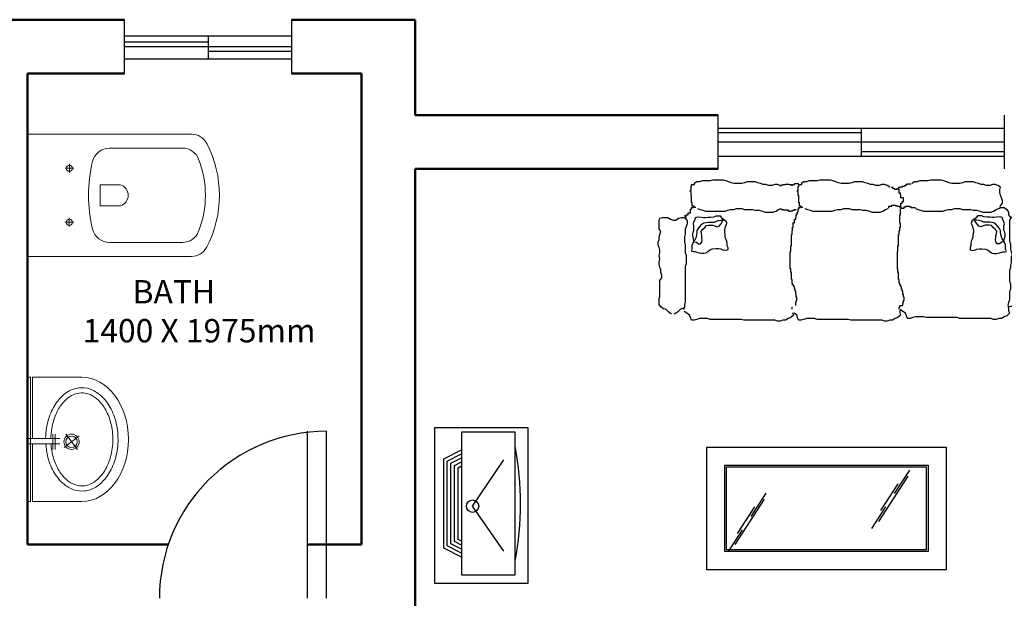
# Model space of a CAD drawing. Units: millimetres. Extents: x -857 to 54106, y -13666 to 13947.
# Tile 20 of 41: x 24413 to 28540, y 10779 to 13204. Entities that reach past the tile are written whole.
import ezdxf

# ---------------------------------------------------------------- set-up
doc = ezdxf.new("R2010")
doc.units = ezdxf.units.MM
for name, color, linetype, lineweight in [('A-AREA-IDEN', 3, 'Continuous', 18), ('A-DOOR', 1, 'Continuous', 25), ('A-FLOR-FIXT', 8, 'Continuous', 18), ('A-FURN', 21, 'Continuous', 18), ('A-GLAZ', 4, 'Continuous', 25), ('A-SANITARY FITTINGS', 25, 'Continuous', 15), ('A-WALL', 7, 'Continuous', 50)]:
    doc.layers.add(name, color=color, linetype=linetype, lineweight=lineweight)
doc.layers.add('TEFRIŞ', color=11, linetype='Continuous')
doc.styles.get("Standard").update_dxf_attribs({"font": 'arial.ttf'})

# ---------------------------------------------------------------- blocks, each defined once
blk = doc.blocks.new('A$C7d9d00ca')
at = {"layer": 'A-SANITARY FITTINGS'}
for p, q in [((0, 0), (-13.78, 0)), ((-13.78, -18.49), (-13.78, 0)), ((0, -18.49), (0, 0)), ((-9.94, -4.23), (-9.94, -5.23)), ((-3.84, -4.24), (-3.84, -5.24)), ((-10.42, -4.72), (-9.43, -4.72)), ((-3.36, -4.73), (-4.34, -4.73)), ((-12.2, -9.27), (-12.2, -17.48)), ((-1.57, -9.27), (-1.57, -17.48))]:
    blk.add_line(p, q, dxfattribs=at)
for points in [[(-8.08, -8.19), (-5.7, -8.19), (-5.7, -8.19), (-5.7, -10.48)], [(-8.08, -8.19), (-8.08, -10.48)]]:
    blk.add_lwpolyline(points, dxfattribs=at)
for centre in [(-9.94, -4.72), (-3.84, -4.73)]:
    blk.add_circle(centre, 0.342, dxfattribs=at)
for centre, radius, start, end in [((-10.24, -9.27), 1.97, 103.8652, 180), ((-6.89, -22.82), 15.93, 76.135, 103.8652), ((-3.54, -9.27), 1.97, 0.0003, 76.135), ((-6.89, -10.13), 1.24, 196.5098, 343.4902), ((-10.24, -17.48), 1.97, 180, 248.6555), ((-3.54, -17.48), 1.97, 291.3447, 0.0003), ((-11.81, -18.49), 1.97, 180, 242.8074), ((-1.97, -18.49), 1.97, 297.1926, 0), ((-6.89, -8.92), 11.16, 248.6555, 291.3447), ((-6.89, -8.92), 12.74, 242.8074, 297.1926)]:
    blk.add_arc(centre, radius, start, end, dxfattribs=at)
blk = doc.blocks.new('A$C0124305E')
at = {"layer": 'A-SANITARY FITTINGS'}
for p, q in [((-8.42, 16.01), (-0.8, 16.01)), ((-0.8, 7.08), (-0.8, 16.01)), ((-5.66, 7.68), (-8, 5.88)), ((-7.73, 7.95), (-5.93, 5.62)), ((-4.31, 5.61), (-4.31, 7.96)), ((-3.91, 5.61), (-3.91, 7.96)), ((0, 7.08), (-4.99, 7.08)), ((0, 6.28), (-4.99, 6.28)), ((-0.8, -3.19), (-0.8, 6.28)), ((-8.42, -3.19), (-0.8, -3.19))]:
    blk.add_line(p, q, dxfattribs=at)
blk.add_lwpolyline([(-0.5, 16.01), (0, 16.01), (0, -3.19), (-0.5, -3.19)], close=True, dxfattribs=at)
for radius in [1.18, 0.885]:
    blk.add_circle((-6.83, 6.78), radius, dxfattribs=at)
at = {"layer": 'A-SANITARY FITTINGS', "extrusion": (0, 0, -1)}
blk.add_ellipse((-8.42, 6.41), major_axis=(0, 9.6), ratio=0.75, start_param=3.141593, end_param=6.283185, dxfattribs=at)
at = {"layer": 'A-SANITARY FITTINGS'}
for points, knots in [([(-2.82, 6.28), (-2.82, 5.74), (-2.87, 5.2), (-3.1, 3.74), (-3.37, 2.86), (-4.09, 1.28), (-4.55, 0.6), (-5.56, -0.5), (-6.12, -0.92), (-7.25, -1.45), (-7.83, -1.58), (-8.98, -1.59), (-9.55, -1.46), (-10.69, -0.93), (-11.25, -0.52), (-12.27, 0.57), (-12.72, 1.25), (-13.45, 2.82), (-13.72, 3.71), (-14.02, 5.56), (-14.05, 6.52), (-13.88, 8.41), (-13.67, 9.32), (-13.04, 10.99), (-12.62, 11.73), (-11.66, 12.96), (-11.12, 13.45), (-10, 14.13), (-9.43, 14.32), (-8.28, 14.45), (-7.7, 14.39), (-6.56, 14), (-5.99, 13.66), (-4.93, 12.71), (-4.44, 12.09), (-3.62, 10.62), (-3.3, 9.78), (-2.96, 8.29), (-2.87, 7.69), (-2.84, 7.08)], [1.58652, 1.58652, 1.58652, 1.58652, 1.780321, 1.780321, 2.120053, 2.120053, 2.459785, 2.459785, 2.799517, 2.799517, 3.139249, 3.139249, 3.478981, 3.478981, 3.818713, 3.818713, 4.158445, 4.158445, 4.498177, 4.498177, 4.837909, 4.837909, 5.177641, 5.177641, 5.517373, 5.517373, 5.857105, 5.857105, 6.196837, 6.196837, 6.536569, 6.536569, 6.876301, 6.876301, 7.216033, 7.216033, 7.555765, 7.555765, 7.774364, 7.774364, 7.774364, 7.774364]), ([(-3.62, 6.29), (-3.62, 5.76), (-3.67, 5.23), (-3.88, 3.96), (-4.1, 3.23), (-4.65, 1.95), (-4.98, 1.39), (-5.72, 0.46), (-6.12, 0.1), (-6.92, -0.44), (-7.32, -0.61), (-8.11, -0.8), (-8.5, -0.81), (-9.28, -0.69), (-9.68, -0.55), (-10.48, -0.08), (-10.89, 0.24), (-11.67, 1.13), (-12.05, 1.7), (-12.66, 3.01), (-12.9, 3.76), (-13.2, 5.38), (-13.25, 6.28), (-13.13, 8.02), (-12.95, 8.88), (-12.42, 10.42), (-12.06, 11.12), (-11.23, 12.25), (-10.77, 12.7), (-9.92, 13.26), (-9.53, 13.43), (-8.78, 13.62), (-8.41, 13.64), (-7.66, 13.54), (-7.28, 13.42), (-6.51, 13.02), (-6.12, 12.73), (-5.35, 11.95), (-4.97, 11.43), (-4.34, 10.23), (-4.08, 9.54), (-3.76, 8.24), (-3.67, 7.64), (-3.63, 7.03)], [1.58652, 1.58652, 1.58652, 1.58652, 1.790653, 1.790653, 2.093007, 2.093007, 2.384527, 2.384527, 2.676047, 2.676047, 2.967567, 2.967567, 3.259087, 3.259087, 3.550608, 3.550608, 3.842128, 3.842128, 4.155456, 4.155456, 4.468784, 4.468784, 4.806699, 4.806699, 5.144614, 5.144614, 5.482529, 5.482529, 5.820444, 5.820444, 6.099515, 6.099515, 6.378586, 6.378586, 6.657656, 6.657656, 6.936727, 6.936727, 7.23864, 7.23864, 7.540552, 7.540552, 7.774364, 7.774364, 7.774364, 7.774364])]:
    blk.add_open_spline(points, degree=3, knots=knots, dxfattribs=at)
blk = doc.blocks.new('27')
at = {"layer": 'TEFRIŞ'}
for p, q in [((-1750.11, -460.72), (-1775.76, -443.38)), ((-1725.16, -443.38), (-1750.11, -460.72))]:
    blk.add_line(p, q, dxfattribs=at)
for points in [[(-1707.18, -481.65), (-1793.65, -481.65), (-1793.65, -429.97), (-1707.18, -429.97)], [(-1791.19, -466.78), (-1711.98, -466.78), (-1711.98, -437.07), (-1791.19, -437.07)]]:
    blk.add_lwpolyline(points, close=True, dxfattribs=at)
for points in [[(-1721.88, -466.78), (-1726.83, -476.68), (-1776.34, -476.68), (-1781.29, -466.78)], [(-1724.1, -466.78), (-1728.06, -474.7), (-1775.12, -474.7), (-1779.08, -466.78)], [(-1726.31, -466.78), (-1729.28, -472.72), (-1773.89, -472.72), (-1776.86, -466.78)], [(-1728.53, -466.78), (-1730.51, -470.74), (-1772.67, -470.74), (-1774.65, -466.78)], [(-1730.74, -466.78), (-1731.73, -468.76), (-1771.44, -468.76), (-1772.43, -466.78)]]:
    blk.add_lwpolyline(points, dxfattribs=at)
blk.add_circle((-1750.11, -460.72), 3.43, dxfattribs=at)
blk.add_arc((-1751.43, -604.56), 170.46, 79.2853, 100.7147, dxfattribs=at)
blk = doc.blocks.new('24')
at = {"layer": 'TEFRIŞ'}
for p, q in [((-1851.9, -153.78), (-1851.9, -152.78)), ((-1851.9, -152.78), (-1850.24, -152.78)), ((-1849.09, -151.25), (-1850.56, -152.23)), ((-1850.24, -152.78), (-1850.24, -152.11)), ((-1847.61, -151.25), (-1849.09, -151.25)), ((-1846.13, -150.75), (-1847.61, -151.25)), ((-1841.7, -150.75), (-1846.13, -150.75)), ((-1840.23, -150.26), (-1841.7, -150.75)), ((-1834.32, -150.26), (-1840.23, -150.26)), ((-1832.84, -150.75), (-1834.32, -150.26)), ((-1831.36, -151.25), (-1832.84, -150.75)), ((-1829.89, -151.74), (-1831.36, -151.25)), ((-1828.41, -152.23), (-1829.89, -151.74)), ((-1823.98, -152.23), (-1828.41, -152.23)), ((-1822.5, -151.74), (-1823.98, -152.23)), ((-1821.03, -151.25), (-1822.5, -151.74)), ((-1816.6, -151.25), (-1821.03, -151.25)), ((-1815.12, -151.74), (-1816.6, -151.25)), ((-1813.64, -152.23), (-1815.12, -151.74)), ((-1812.17, -152.72), (-1813.64, -152.23)), ((-1810.69, -152.72), (-1812.17, -152.72)), ((-1809.21, -153.21), (-1810.69, -152.72)), ((-1805.77, -152.72), (-1807.24, -153.21)), ((-1804.29, -152.72), (-1805.77, -152.72)), ((-1802.81, -153.21), (-1804.29, -152.72)), ((-1801, -152.88), (-1801, -152.68)), ((-1801, -152.68), (-1800, -152.68)), ((-1800, -152.68), (-1800, -152.48)), ((-1800, -152.48), (-1797.79, -152.48)), ((-1797.79, -152.48), (-1797.79, -152.68)), ((-1797.79, -152.68), (-1796.79, -152.68)), ((-1796.79, -152.68), (-1796.79, -153.08)), ((-1795.78, -153.08), (-1795.78, -152.68)), ((-1795.78, -152.68), (-1794.78, -152.68)), ((-1794.78, -152.68), (-1794.78, -152.08)), ((-1794.78, -152.08), (-1792.77, -152.08)), ((-1792.77, -152.08), (-1792.77, -152.68)), ((-1792.77, -152.68), (-1792.57, -152.68)), ((-1792.5, -152.78), (-1790.84, -152.78)), ((-1792.5, -153.78), (-1792.5, -152.78)), ((-1789.69, -151.25), (-1791.16, -152.23)), ((-1790.84, -152.78), (-1790.84, -152.11)), ((-1788.21, -151.25), (-1789.69, -151.25)), ((-1786.73, -150.75), (-1788.21, -151.25)), ((-1782.3, -150.75), (-1786.73, -150.75)), ((-1780.83, -150.26), (-1782.3, -150.75)), ((-1774.92, -150.26), (-1780.83, -150.26)), ((-1773.44, -150.75), (-1774.92, -150.26)), ((-1771.96, -151.25), (-1773.44, -150.75)), ((-1770.49, -151.74), (-1771.96, -151.25)), ((-1769.01, -152.23), (-1770.49, -151.74)), ((-1764.58, -152.23), (-1769.01, -152.23)), ((-1763.1, -151.74), (-1764.58, -152.23)), ((-1761.63, -151.25), (-1763.1, -151.74)), ((-1757.2, -151.25), (-1761.63, -151.25)), ((-1755.72, -151.74), (-1757.2, -151.25)), ((-1754.24, -152.23), (-1755.72, -151.74)), ((-1752.77, -152.72), (-1754.24, -152.23)), ((-1751.29, -152.72), (-1752.77, -152.72)), ((-1749.81, -153.21), (-1751.29, -152.72)), ((-1746.37, -152.72), (-1747.84, -153.21)), ((-1744.89, -152.72), (-1746.37, -152.72)), ((-1743.41, -153.21), (-1744.89, -152.72)), ((-1733.14, -152.78), (-1733.14, -153.45)), ((-1732.14, -152.78), (-1733.14, -152.78)), ((-1732.14, -152.45), (-1732.14, -152.78)), ((-1730.14, -152.45), (-1732.14, -152.45)), ((-1728.32, -151.25), (-1729.8, -152.23)), ((-1726.85, -151.25), (-1728.32, -151.25)), ((-1725.37, -150.75), (-1726.85, -151.25)), ((-1720.94, -150.75), (-1725.37, -150.75)), ((-1719.46, -150.26), (-1720.94, -150.75)), ((-1713.56, -150.26), (-1719.46, -150.26)), ((-1712.08, -150.75), (-1713.56, -150.26)), ((-1710.6, -151.25), (-1712.08, -150.75)), ((-1709.12, -151.74), (-1710.6, -151.25)), ((-1707.65, -152.23), (-1709.12, -151.74)), ((-1703.22, -152.23), (-1707.65, -152.23)), ((-1701.74, -151.74), (-1703.22, -152.23)), ((-1700.26, -151.25), (-1701.74, -151.74)), ((-1695.83, -151.25), (-1700.26, -151.25)), ((-1694.36, -151.74), (-1695.83, -151.25)), ((-1692.88, -152.23), (-1694.36, -151.74)), ((-1691.4, -152.72), (-1692.88, -152.23)), ((-1689.93, -152.72), (-1691.4, -152.72)), ((-1688.45, -153.21), (-1689.93, -152.72)), ((-1685, -152.72), (-1686.48, -153.21)), ((-1683.53, -152.72), (-1685, -152.72)), ((-1682.05, -153.21), (-1683.53, -152.72)), ((-1852.57, -156.78), (-1852.57, -155.78)), ((-1852.57, -155.78), (-1852.24, -155.78)), ((-1852.24, -156.78), (-1852.57, -156.78)), ((-1852.24, -155.78), (-1852.24, -153.78)), ((-1852.24, -153.78), (-1851.9, -153.78)), ((-1852.24, -158.78), (-1852.24, -156.78)), ((-1807.24, -153.21), (-1809.21, -153.21)), ((-1803.01, -153.28), (-1802.01, -153.28)), ((-1802.01, -153.28), (-1802.01, -152.88)), ((-1802.01, -152.88), (-1801, -152.88)), ((-1796.79, -153.08), (-1795.78, -153.08)), ((-1793.17, -155.78), (-1792.84, -155.78)), ((-1793.17, -156.78), (-1793.17, -155.78)), ((-1792.84, -156.78), (-1793.17, -156.78)), ((-1792.84, -155.78), (-1792.84, -153.78)), ((-1792.84, -153.78), (-1792.5, -153.78)), ((-1792.84, -158.78), (-1792.84, -156.78)), ((-1747.84, -153.21), (-1749.81, -153.21)), ((-1741.94, -154.2), (-1743.41, -153.21)), ((-1741.14, -154.45), (-1741.14, -154.11)), ((-1740.14, -154.45), (-1741.14, -154.45)), ((-1740.14, -155.11), (-1740.14, -154.45)), ((-1739.14, -155.11), (-1740.14, -155.11)), ((-1739.14, -155.45), (-1739.14, -155.11)), ((-1738.14, -155.45), (-1739.14, -155.45)), ((-1738.14, -155.11), (-1738.14, -155.45)), ((-1737.14, -155.11), (-1738.14, -155.11)), ((-1737.14, -154.45), (-1737.14, -155.11)), ((-1736.14, -154.45), (-1737.14, -154.45)), ((-1737.14, -155.45), (-1737.14, -155.11)), ((-1736.81, -155.45), (-1737.14, -155.45)), ((-1736.81, -157.45), (-1736.81, -155.45)), ((-1736.14, -157.45), (-1736.81, -157.45)), ((-1735.14, -154.11), (-1736.14, -154.11)), ((-1736.14, -154.11), (-1736.14, -154.45)), ((-1736.14, -158.45), (-1736.14, -157.45)), ((-1735.14, -153.78), (-1735.14, -154.11)), ((-1734.14, -153.78), (-1735.14, -153.78)), ((-1734.14, -153.45), (-1734.14, -153.78)), ((-1733.14, -153.45), (-1734.14, -153.45)), ((-1686.48, -153.21), (-1688.45, -153.21)), ((-1680.57, -154.2), (-1682.05, -153.21)), ((-1681.06, -155.67), (-1680.57, -154.2)), ((-1681.06, -157.15), (-1681.06, -155.67)), ((-1680.57, -158.63), (-1681.06, -157.15)), ((-1851.9, -158.78), (-1852.24, -158.78)), ((-1851.9, -162.78), (-1851.9, -158.78)), ((-1851.57, -162.78), (-1851.9, -162.78)), ((-1851.57, -164.78), (-1851.57, -162.78)), ((-1792.5, -158.78), (-1792.84, -158.78)), ((-1792.5, -162.78), (-1792.5, -158.78)), ((-1792.17, -162.78), (-1792.5, -162.78)), ((-1792.17, -164.78), (-1792.17, -162.78)), ((-1735.81, -158.45), (-1736.14, -158.45)), ((-1735.81, -160.11), (-1735.81, -158.45)), ((-1734.48, -160.11), (-1735.81, -160.11)), ((-1735.81, -163.11), (-1735.14, -163.11)), ((-1735.81, -165.11), (-1735.81, -163.11)), ((-1735.14, -162.11), (-1734.48, -162.11)), ((-1735.14, -163.11), (-1735.14, -162.11)), ((-1734.48, -162.11), (-1734.48, -160.11)), ((-1680.08, -160.1), (-1680.57, -158.63)), ((-1680.57, -164.53), (-1679.59, -163.05)), ((-1679.59, -161.58), (-1680.08, -160.1)), ((-1679.59, -163.05), (-1679.59, -161.58)), ((-1853.9, -169.44), (-1853.9, -168.44)), ((-1853.9, -168.44), (-1852.57, -168.44)), ((-1852.57, -168.44), (-1852.57, -166.44)), ((-1852.57, -166.44), (-1851.9, -166.44)), ((-1851.9, -166.44), (-1851.9, -165.44)), ((-1851.9, -165.44), (-1850.9, -165.44)), ((-1850.57, -164.78), (-1851.57, -164.78)), ((-1850.9, -165.44), (-1850.9, -164.78)), ((-1850.57, -165.44), (-1850.57, -164.78)), ((-1849.57, -165.44), (-1850.57, -165.44)), ((-1848.59, -166), (-1847.12, -166.5)), ((-1847.12, -166.5), (-1845.64, -166.99)), ((-1845.64, -166.99), (-1844.16, -167.48)), ((-1844.16, -167.48), (-1833.33, -167.48)), ((-1833.33, -167.48), (-1831.86, -166.99)), ((-1831.86, -166.99), (-1830.38, -166.5)), ((-1830.38, -166.5), (-1828.41, -166.5)), ((-1828.41, -166.5), (-1826.93, -166)), ((-1826.93, -166), (-1823.98, -166)), ((-1823.98, -166), (-1822.5, -166.5)), ((-1822.5, -166.5), (-1818.07, -166.5)), ((-1818.07, -166.5), (-1816.6, -166.99)), ((-1816.6, -166.99), (-1814.63, -166.99)), ((-1814.63, -166.99), (-1812.66, -167.48)), ((-1812.66, -167.48), (-1811.18, -167.97)), ((-1811.18, -167.97), (-1806.75, -167.97)), ((-1806.75, -167.97), (-1805.27, -167.48)), ((-1805.27, -167.48), (-1803.8, -166.5)), ((-1803.8, -166.5), (-1802.32, -166)), ((-1802.41, -166.32), (-1802.41, -165.92)), ((-1802.01, -166.32), (-1802.41, -166.32)), ((-1802.01, -166.72), (-1802.01, -166.32)), ((-1801, -166.72), (-1802.01, -166.72)), ((-1801, -166.92), (-1801, -166.72)), ((-1798.99, -166.92), (-1801, -166.92)), ((-1798.99, -167.12), (-1798.99, -166.92)), ((-1797.99, -167.12), (-1798.99, -167.12)), ((-1797.99, -167.72), (-1797.99, -167.12)), ((-1796.99, -167.72), (-1797.99, -167.72)), ((-1795.98, -167.52), (-1796.99, -167.52)), ((-1796.99, -167.52), (-1796.99, -167.72)), ((-1794.98, -167.12), (-1795.98, -167.12)), ((-1795.98, -167.12), (-1795.98, -167.52)), ((-1793.98, -166.72), (-1794.98, -166.72)), ((-1794.98, -166.72), (-1794.98, -167.12)), ((-1793.78, -169.93), (-1793.78, -168.92)), ((-1793.78, -168.92), (-1793.18, -168.92)), ((-1793.18, -168.92), (-1793.18, -167.92)), ((-1793.18, -167.92), (-1792.77, -167.92)), ((-1793.17, -166.44), (-1792.5, -166.44)), ((-1792.77, -167.92), (-1792.77, -166.32)), ((-1792.5, -165.44), (-1791.5, -165.44)), ((-1792.5, -166.44), (-1792.5, -165.44)), ((-1791.17, -164.78), (-1792.17, -164.78)), ((-1791.5, -165.44), (-1791.5, -164.78)), ((-1791.17, -165.44), (-1791.17, -164.78)), ((-1790.17, -165.44), (-1791.17, -165.44)), ((-1789.19, -166), (-1787.72, -166.5)), ((-1787.72, -166.5), (-1786.24, -166.99)), ((-1786.24, -166.99), (-1784.76, -167.48)), ((-1784.76, -167.48), (-1773.93, -167.48)), ((-1773.93, -167.48), (-1772.46, -166.99)), ((-1772.46, -166.99), (-1770.98, -166.5)), ((-1770.98, -166.5), (-1769.01, -166.5)), ((-1769.01, -166.5), (-1767.53, -166)), ((-1767.53, -166), (-1764.58, -166)), ((-1764.58, -166), (-1763.1, -166.5)), ((-1763.1, -166.5), (-1758.67, -166.5)), ((-1758.67, -166.5), (-1757.2, -166.99)), ((-1757.2, -166.99), (-1755.23, -166.99)), ((-1755.23, -166.99), (-1753.26, -167.48)), ((-1753.26, -167.48), (-1751.78, -167.97)), ((-1751.78, -167.97), (-1747.35, -167.97)), ((-1747.35, -167.97), (-1745.87, -167.48)), ((-1745.87, -167.48), (-1744.4, -166.5)), ((-1744.4, -166.5), (-1742.92, -166)), ((-1742.48, -164.78), (-1740.81, -164.78)), ((-1742.48, -165.78), (-1742.48, -164.78)), ((-1740.81, -164.11), (-1738.81, -164.11)), ((-1740.81, -164.78), (-1740.81, -164.11)), ((-1738.81, -164.11), (-1738.81, -164.45)), ((-1738.81, -164.45), (-1737.81, -164.45)), ((-1737.81, -164.45), (-1737.81, -164.78)), ((-1737.81, -164.78), (-1736.81, -164.78)), ((-1736.81, -164.78), (-1736.81, -165.11)), ((-1736.81, -165.11), (-1735.81, -165.11)), ((-1735.81, -165.44), (-1736.14, -165.44)), ((-1736.14, -165.78), (-1734.14, -165.78)), ((-1736.14, -166.11), (-1735.81, -166.11)), ((-1736.14, -169.44), (-1736.14, -166.11)), ((-1735.81, -165.11), (-1735.81, -165.44)), ((-1734.14, -165.11), (-1733.14, -165.11)), ((-1734.14, -165.78), (-1734.14, -165.11)), ((-1733.14, -164.78), (-1731.14, -164.78)), ((-1733.14, -165.11), (-1733.14, -164.78)), ((-1731.14, -164.78), (-1731.14, -165.11)), ((-1731.14, -165.11), (-1730.14, -165.11)), ((-1730.14, -165.11), (-1730.14, -165.44)), ((-1730.14, -165.44), (-1727.81, -165.44)), ((-1727.83, -166), (-1726.35, -166.5)), ((-1726.35, -166.5), (-1724.88, -166.99)), ((-1724.88, -166.99), (-1723.4, -167.48)), ((-1723.4, -167.48), (-1712.57, -167.48)), ((-1712.57, -167.48), (-1711.09, -166.99)), ((-1711.09, -166.99), (-1709.62, -166.5)), ((-1709.62, -166.5), (-1707.65, -166.5)), ((-1707.65, -166.5), (-1706.17, -166)), ((-1706.17, -166), (-1703.22, -166)), ((-1703.22, -166), (-1701.74, -166.5)), ((-1701.74, -166.5), (-1697.31, -166.5)), ((-1697.31, -166.5), (-1695.83, -166.99)), ((-1695.83, -166.99), (-1693.86, -166.99)), ((-1693.86, -166.99), (-1691.89, -167.48)), ((-1691.89, -167.48), (-1690.42, -167.97)), ((-1690.42, -167.97), (-1685.99, -167.97)), ((-1685.99, -167.97), (-1684.51, -167.48)), ((-1684.51, -167.48), (-1683.03, -166.5)), ((-1683.03, -166.5), (-1681.56, -166)), ((-1681.56, -166), (-1680.08, -165.51)), ((-1681.06, -166), (-1680.57, -164.53)), ((-1680.08, -165.51), (-1678.6, -165.51)), ((-1678.6, -165.51), (-1677.13, -166.5)), ((-1677.13, -166.5), (-1676.14, -167.97)), ((-1676.14, -167.97), (-1676.14, -169.45)), ((-1869.99, -172.89), (-1869.5, -171.42)), ((-1869.99, -177.32), (-1869.99, -172.89)), ((-1869.5, -171.42), (-1868.02, -170.92)), ((-1868.02, -170.92), (-1865.07, -170.92)), ((-1865.07, -170.92), (-1863.59, -171.91)), ((-1863.59, -171.91), (-1862.11, -172.4)), ((-1862.11, -172.4), (-1860.63, -172.4)), ((-1860.63, -172.4), (-1859.16, -171.42)), ((-1859.16, -171.42), (-1857.68, -170.92)), ((-1857.68, -170.92), (-1856.2, -170.92)), ((-1856.2, -170.92), (-1854.73, -171.42)), ((-1855.22, -171.42), (-1855.71, -169.94)), ((-1854.24, -172.89), (-1855.22, -171.42)), ((-1854.9, -169.44), (-1853.9, -169.44)), ((-1854.9, -170.78), (-1854.9, -169.44)), ((-1854.73, -175.84), (-1854.24, -174.37)), ((-1854.24, -174.37), (-1854.24, -172.89)), ((-1850.85, -174.48), (-1850.62, -173.32)), ((-1850.62, -175.64), (-1850.85, -174.48)), ((-1850.62, -173.32), (-1849.92, -172.16)), ((-1849.92, -172.16), (-1849.69, -171)), ((-1849.69, -171), (-1848.53, -170.54)), ((-1848.53, -170.54), (-1846.44, -170.77)), ((-1847.14, -175.87), (-1846.21, -174.71)), ((-1846.44, -170.77), (-1845.28, -171)), ((-1846.21, -174.71), (-1845.05, -174.01)), ((-1845.28, -171), (-1844.12, -171)), ((-1845.05, -174.01), (-1843.89, -173.78)), ((-1844.12, -171), (-1842.73, -170.77)), ((-1843.89, -173.78), (-1842.73, -173.55)), ((-1842.73, -170.77), (-1841.34, -170.77)), ((-1842.73, -173.55), (-1839.25, -173.55)), ((-1841.34, -170.77), (-1839.48, -170.54)), ((-1839.48, -170.54), (-1838.32, -170.07)), ((-1839.25, -173.55), (-1838.09, -173.09)), ((-1838.32, -170.07), (-1836, -170.07)), ((-1838.09, -173.09), (-1836.93, -172.62)), ((-1836.93, -172.62), (-1835.54, -172.39)), ((-1836.7, -175.87), (-1835.77, -174.71)), ((-1836, -170.07), (-1835.31, -171.23)), ((-1835.77, -174.71), (-1835.08, -173.55)), ((-1835.54, -172.39), (-1834.38, -172.16)), ((-1835.31, -171.23), (-1833.92, -172.16)), ((-1835.08, -173.55), (-1834.38, -172.39)), ((-1834.38, -172.39), (-1834.15, -171.93)), ((-1833.92, -172.16), (-1832.76, -173.09)), ((-1832.52, -174.25), (-1832.99, -175.4)), ((-1832.76, -173.09), (-1832.52, -174.25)), ((-1795.54, -174.11), (-1795.88, -174.11)), ((-1795.78, -173.94), (-1794.78, -173.94)), ((-1795.54, -176.44), (-1795.54, -174.11)), ((-1794.78, -173.94), (-1794.78, -171.93)), ((-1794.78, -171.93), (-1794.18, -171.93)), ((-1794.18, -171.93), (-1794.18, -170.93)), ((-1794.18, -170.93), (-1793.98, -170.93)), ((-1793.98, -170.93), (-1793.98, -169.93)), ((-1793.98, -169.93), (-1793.78, -169.93)), ((-1736.48, -174.11), (-1736.48, -169.44)), ((-1736.48, -169.44), (-1736.14, -169.44)), ((-1736.14, -174.11), (-1736.48, -174.11)), ((-1736.14, -176.44), (-1736.14, -174.11)), ((-1696.59, -173.09), (-1696.83, -174.25)), ((-1696.83, -174.25), (-1696.36, -175.4)), ((-1695.43, -172.16), (-1696.59, -173.09)), ((-1694.04, -171.23), (-1695.43, -172.16)), ((-1694.97, -172.39), (-1695.2, -171.93)), ((-1693.81, -172.39), (-1694.97, -172.16)), ((-1694.27, -173.55), (-1694.97, -172.39)), ((-1693.58, -174.71), (-1694.27, -173.55)), ((-1693.35, -170.07), (-1694.04, -171.23)), ((-1692.42, -172.62), (-1693.81, -172.39)), ((-1692.65, -175.87), (-1693.58, -174.71)), ((-1691.03, -170.07), (-1693.35, -170.07)), ((-1691.26, -173.09), (-1692.42, -172.62)), ((-1690.1, -173.55), (-1691.26, -173.09)), ((-1689.87, -170.54), (-1691.03, -170.07)), ((-1686.62, -173.55), (-1690.1, -173.55)), ((-1688.01, -170.77), (-1689.87, -170.54)), ((-1686.62, -170.77), (-1688.01, -170.77)), ((-1685.23, -171), (-1686.62, -170.77)), ((-1685.46, -173.78), (-1686.62, -173.55)), ((-1684.3, -174.01), (-1685.46, -173.78)), ((-1684.07, -171), (-1685.23, -171)), ((-1683.14, -174.71), (-1684.3, -174.01)), ((-1682.91, -170.77), (-1684.07, -171)), ((-1682.21, -175.87), (-1683.14, -174.71)), ((-1680.82, -170.54), (-1682.91, -170.77)), ((-1679.66, -171), (-1680.82, -170.54)), ((-1679.43, -172.16), (-1679.66, -171)), ((-1678.73, -173.32), (-1679.43, -172.16)), ((-1678.5, -174.48), (-1678.73, -173.32)), ((-1678.73, -175.64), (-1678.5, -174.48)), ((-1676.14, -169.45), (-1675.16, -170.92)), ((-1674.66, -170.92), (-1675.65, -172.4)), ((-1675.65, -172.4), (-1675.65, -184.21)), ((-1673.19, -170.43), (-1674.66, -170.92)), ((-1671.22, -170.43), (-1673.19, -170.43)), ((-1669.74, -170.92), (-1671.22, -170.43)), ((-1668.27, -171.42), (-1669.74, -170.92)), ((-1664.33, -171.42), (-1668.27, -171.42)), ((-1662.85, -170.43), (-1664.33, -171.42)), ((-1661.37, -170.92), (-1662.85, -170.43)), ((-1659.9, -171.91), (-1661.37, -170.92)), ((-1659.9, -173.38), (-1659.9, -171.91)), ((-1658.91, -176.34), (-1659.9, -173.38)), ((-1869, -178.8), (-1869.99, -177.32)), ((-1869.99, -181.75), (-1869, -178.8)), ((-1855.22, -177.32), (-1854.73, -175.84)), ((-1855.22, -180.27), (-1855.22, -177.32)), ((-1851.31, -180.27), (-1851.08, -179.11)), ((-1851.08, -179.11), (-1850.62, -177.95)), ((-1850.62, -177.95), (-1850.62, -175.64)), ((-1848.99, -180.5), (-1848.76, -179.35)), ((-1848.76, -178.19), (-1848.07, -177.03)), ((-1848.76, -179.35), (-1848.76, -178.19)), ((-1848.07, -177.03), (-1847.14, -175.87)), ((-1846.67, -178.65), (-1845.75, -177.49)), ((-1846.44, -179.81), (-1846.67, -178.65)), ((-1846.21, -180.97), (-1846.44, -179.81)), ((-1845.75, -177.49), (-1844.59, -176.56)), ((-1844.59, -176.56), (-1843.66, -175.4)), ((-1843.66, -175.4), (-1842.5, -175.17)), ((-1842.5, -175.17), (-1840.18, -175.17)), ((-1840.18, -175.17), (-1839.02, -175.64)), ((-1839.02, -175.64), (-1837.86, -176.1)), ((-1837.86, -176.1), (-1836.7, -175.87)), ((-1833.45, -176.8), (-1833.68, -178.19)), ((-1833.68, -178.19), (-1833.68, -179.35)), ((-1833.68, -179.35), (-1833.45, -180.5)), ((-1832.99, -175.4), (-1833.45, -176.8)), ((-1796.21, -180.44), (-1796.21, -178.44)), ((-1796.21, -178.44), (-1795.88, -178.44)), ((-1795.88, -178.44), (-1795.88, -176.44)), ((-1795.88, -176.44), (-1795.54, -176.44)), ((-1736.81, -178.44), (-1736.48, -178.44)), ((-1736.81, -180.44), (-1736.81, -178.44)), ((-1736.48, -178.44), (-1736.48, -176.44)), ((-1736.48, -176.44), (-1736.14, -176.44)), ((-1696.36, -175.4), (-1695.9, -176.8)), ((-1695.9, -176.8), (-1695.67, -178.19)), ((-1695.67, -179.35), (-1695.9, -180.5)), ((-1695.67, -178.19), (-1695.67, -179.35)), ((-1691.49, -176.1), (-1692.65, -175.87)), ((-1690.33, -175.64), (-1691.49, -176.1)), ((-1689.17, -175.17), (-1690.33, -175.64)), ((-1686.85, -175.17), (-1689.17, -175.17)), ((-1685.69, -175.4), (-1686.85, -175.17)), ((-1684.76, -176.56), (-1685.69, -175.4)), ((-1683.6, -177.49), (-1684.76, -176.56)), ((-1682.68, -178.65), (-1683.6, -177.49)), ((-1683.14, -180.97), (-1682.91, -179.81)), ((-1682.91, -179.81), (-1682.68, -178.65)), ((-1681.28, -177.03), (-1682.21, -175.87)), ((-1680.59, -178.19), (-1681.28, -177.03)), ((-1680.59, -179.35), (-1680.59, -178.19)), ((-1680.36, -180.5), (-1680.59, -179.35)), ((-1678.73, -177.95), (-1678.73, -175.64)), ((-1678.27, -179.11), (-1678.73, -177.95)), ((-1678.04, -180.27), (-1678.27, -179.11)), ((-1659.4, -180.76), (-1658.91, -179.29)), ((-1658.91, -179.29), (-1658.91, -176.34)), ((-1870.48, -184.7), (-1869.99, -183.22)), ((-1870.48, -186.17), (-1870.48, -184.7)), ((-1869.99, -183.22), (-1869.99, -181.75)), ((-1855.71, -181.75), (-1855.22, -180.27)), ((-1855.71, -184.7), (-1855.71, -181.75)), ((-1855.22, -186.17), (-1855.71, -184.7)), ((-1851.55, -186.07), (-1850.85, -184.91)), ((-1851.31, -181.43), (-1851.31, -180.27)), ((-1850.85, -182.59), (-1851.31, -181.43)), ((-1850.62, -183.75), (-1850.85, -182.59)), ((-1850.85, -184.91), (-1850.62, -183.75)), ((-1850.39, -183.98), (-1849.69, -182.82)), ((-1850.39, -184.45), (-1849.23, -184.68)), ((-1849.69, -182.82), (-1849.23, -181.66)), ((-1849.23, -181.66), (-1848.99, -180.5)), ((-1849.23, -184.68), (-1848.07, -185.6)), ((-1848.07, -185.6), (-1846.91, -185.6)), ((-1846.91, -185.6), (-1846.21, -184.45)), ((-1846.21, -182.13), (-1846.21, -180.97)), ((-1845.98, -183.29), (-1846.21, -182.13)), ((-1846.21, -184.45), (-1845.98, -183.29)), ((-1833.45, -180.5), (-1833.45, -181.9)), ((-1833.45, -181.9), (-1832.99, -183.05)), ((-1832.99, -183.05), (-1832.52, -184.21)), ((-1832.52, -184.21), (-1832.29, -185.37)), ((-1832.29, -185.37), (-1832.29, -186.53)), ((-1796.54, -186.77), (-1796.54, -180.44)), ((-1796.54, -180.44), (-1796.21, -180.44)), ((-1737.14, -180.44), (-1736.81, -180.44)), ((-1737.14, -186.77), (-1737.14, -180.44)), ((-1696.83, -184.21), (-1697.06, -185.37)), ((-1697.06, -185.37), (-1697.06, -186.53)), ((-1696.36, -183.05), (-1696.83, -184.21)), ((-1695.9, -181.9), (-1696.36, -183.05)), ((-1695.9, -180.5), (-1695.9, -181.9)), ((-1683.37, -183.29), (-1683.14, -182.13)), ((-1683.14, -184.45), (-1683.37, -183.29)), ((-1683.14, -182.13), (-1683.14, -180.97)), ((-1682.44, -185.6), (-1683.14, -184.45)), ((-1681.28, -185.6), (-1682.44, -185.6)), ((-1680.12, -184.68), (-1681.28, -185.6)), ((-1680.12, -181.66), (-1680.36, -180.5)), ((-1679.66, -182.82), (-1680.12, -181.66)), ((-1678.97, -184.45), (-1680.12, -184.68)), ((-1678.97, -183.98), (-1679.66, -182.82)), ((-1678.73, -183.75), (-1678.5, -182.59)), ((-1678.5, -184.91), (-1678.73, -183.75)), ((-1678.5, -182.59), (-1678.04, -181.43)), ((-1677.81, -186.07), (-1678.5, -184.91)), ((-1678.04, -181.43), (-1678.04, -180.27)), ((-1675.65, -184.21), (-1675.16, -185.68)), ((-1659.4, -183.71), (-1659.4, -180.76)), ((-1658.91, -185.19), (-1659.4, -183.71)), ((-1658.91, -188.14), (-1658.91, -185.19)), ((-1869.99, -187.65), (-1870.48, -186.17)), ((-1869.5, -189.13), (-1869.99, -187.65)), ((-1869.99, -192.08), (-1869.5, -190.6)), ((-1869.5, -190.6), (-1869.5, -189.13)), ((-1855.22, -190.6), (-1855.22, -186.17)), ((-1854.73, -192.08), (-1855.22, -190.6)), ((-1851.08, -190.01), (-1852.01, -189.78)), ((-1851.78, -189.54), (-1851.55, -188.39)), ((-1851.55, -188.39), (-1851.55, -186.07)), ((-1849.92, -190.01), (-1851.08, -190.01)), ((-1848.76, -190.47), (-1849.92, -190.01)), ((-1847.6, -190.7), (-1848.76, -190.47)), ((-1846.44, -190.94), (-1847.6, -190.7)), ((-1845.28, -190.94), (-1846.44, -190.94)), ((-1844.12, -190.7), (-1845.28, -190.94)), ((-1842.96, -190.01), (-1844.12, -190.7)), ((-1841.8, -189.08), (-1842.96, -190.01)), ((-1840.64, -188.62), (-1841.8, -189.08)), ((-1838.32, -188.39), (-1840.64, -188.62)), ((-1836.93, -188.39), (-1838.32, -188.39)), ((-1835.54, -188.62), (-1836.93, -188.39)), ((-1834.38, -189.08), (-1835.54, -188.62)), ((-1832.99, -189.31), (-1834.38, -189.08)), ((-1831.83, -188.85), (-1832.99, -189.31)), ((-1832.29, -186.53), (-1831.83, -187.69)), ((-1831.83, -187.69), (-1831.83, -188.85)), ((-1797.21, -199.44), (-1797.21, -189.77)), ((-1797.21, -189.77), (-1796.88, -189.77)), ((-1796.88, -189.77), (-1796.88, -186.77)), ((-1796.88, -186.77), (-1796.54, -186.77)), ((-1737.81, -189.77), (-1737.48, -189.77)), ((-1737.81, -199.44), (-1737.81, -189.77)), ((-1737.48, -186.77), (-1737.14, -186.77)), ((-1737.48, -189.77), (-1737.48, -186.77)), ((-1697.06, -186.53), (-1697.52, -187.69)), ((-1697.52, -187.69), (-1697.52, -188.85)), ((-1697.52, -188.85), (-1696.36, -189.31)), ((-1696.36, -189.31), (-1694.97, -189.08)), ((-1694.97, -189.08), (-1693.81, -188.62)), ((-1693.81, -188.62), (-1692.42, -188.39)), ((-1692.42, -188.39), (-1691.03, -188.39)), ((-1691.03, -188.39), (-1688.71, -188.62)), ((-1688.71, -188.62), (-1687.55, -189.08)), ((-1687.55, -189.08), (-1686.39, -190.01)), ((-1686.39, -190.01), (-1685.23, -190.7)), ((-1685.23, -190.7), (-1684.07, -190.94)), ((-1684.07, -190.94), (-1682.91, -190.94)), ((-1682.91, -190.94), (-1681.75, -190.7)), ((-1681.75, -190.7), (-1680.59, -190.47)), ((-1680.59, -190.47), (-1679.43, -190.01)), ((-1679.43, -190.01), (-1678.27, -190.01)), ((-1678.27, -190.01), (-1677.34, -189.78)), ((-1677.81, -188.39), (-1677.81, -186.07)), ((-1677.57, -189.54), (-1677.81, -188.39)), ((-1675.16, -185.68), (-1675.16, -188.63)), ((-1675.16, -188.63), (-1674.66, -190.11)), ((-1674.66, -190.11), (-1674.17, -191.59)), ((-1659.4, -189.62), (-1658.91, -188.14)), ((-1659.4, -192.57), (-1659.4, -189.62)), ((-1869.5, -194.05), (-1869.99, -192.08)), ((-1869.99, -195.52), (-1869.5, -194.05)), ((-1869.99, -197), (-1869.99, -195.52)), ((-1855.22, -197.98), (-1854.73, -196.51)), ((-1854.73, -196.51), (-1854.73, -192.08)), ((-1674.66, -196.01), (-1675.16, -197.49)), ((-1674.17, -191.59), (-1674.66, -193.06)), ((-1674.66, -193.06), (-1674.66, -196.01)), ((-1659.9, -194.05), (-1659.4, -192.57)), ((-1659.9, -195.52), (-1659.9, -194.05)), ((-1659.4, -197), (-1659.9, -195.52)), ((-1869.5, -198.47), (-1869.99, -197)), ((-1869, -199.95), (-1869.5, -198.47)), ((-1869, -201.43), (-1869, -199.95)), ((-1868.51, -202.9), (-1869, -201.43)), ((-1855.22, -217.66), (-1855.22, -197.98)), ((-1796.88, -199.44), (-1797.21, -199.44)), ((-1796.88, -201.44), (-1796.88, -199.44)), ((-1796.54, -201.44), (-1796.88, -201.44)), ((-1796.54, -205.44), (-1796.54, -201.44)), ((-1737.48, -199.44), (-1737.81, -199.44)), ((-1737.48, -201.44), (-1737.48, -199.44)), ((-1737.14, -201.44), (-1737.48, -201.44)), ((-1737.14, -205.44), (-1737.14, -201.44)), ((-1675.16, -198.97), (-1675.65, -200.44)), ((-1675.65, -200.44), (-1675.65, -206.34)), ((-1675.16, -197.49), (-1675.16, -198.97)), ((-1660.39, -203.39), (-1659.9, -201.92)), ((-1659.9, -201.92), (-1658.91, -200.44)), ((-1658.91, -198.47), (-1659.4, -197)), ((-1658.91, -200.44), (-1658.91, -198.47)), ((-1869.5, -205.85), (-1868.51, -204.38)), ((-1869.5, -214.71), (-1869.5, -205.85)), ((-1868.51, -204.38), (-1868.51, -202.9)), ((-1796.21, -205.44), (-1796.54, -205.44)), ((-1796.21, -207.44), (-1796.21, -205.44)), ((-1795.88, -207.44), (-1796.21, -207.44)), ((-1795.88, -208.44), (-1795.88, -207.44)), ((-1736.81, -205.44), (-1737.14, -205.44)), ((-1736.81, -207.44), (-1736.81, -205.44)), ((-1736.48, -207.44), (-1736.81, -207.44)), ((-1736.48, -208.44), (-1736.48, -207.44)), ((-1675.65, -206.34), (-1675.16, -207.82)), ((-1661.87, -206.34), (-1660.88, -204.87)), ((-1660.88, -207.82), (-1661.87, -206.34)), ((-1660.88, -204.87), (-1660.39, -203.39)), ((-1795.21, -208.44), (-1795.88, -208.44)), ((-1795.21, -209.44), (-1795.21, -208.44)), ((-1794.88, -209.44), (-1795.21, -209.44)), ((-1794.88, -210.77), (-1794.88, -209.44)), ((-1794.54, -210.77), (-1794.88, -210.77)), ((-1794.54, -211.77), (-1794.54, -210.77)), ((-1794.21, -211.77), (-1794.54, -211.77)), ((-1794.21, -213.77), (-1794.21, -211.77)), ((-1735.81, -208.44), (-1736.48, -208.44)), ((-1735.81, -209.44), (-1735.81, -208.44)), ((-1735.48, -209.44), (-1735.81, -209.44)), ((-1735.48, -210.77), (-1735.48, -209.44)), ((-1735.14, -210.77), (-1735.48, -210.77)), ((-1735.14, -211.77), (-1735.14, -210.77)), ((-1734.81, -211.77), (-1735.14, -211.77)), ((-1734.81, -213.77), (-1734.81, -211.77)), ((-1675.16, -210.77), (-1675.65, -212.25)), ((-1675.65, -212.25), (-1675.65, -216.68)), ((-1675.16, -207.82), (-1675.16, -210.77)), ((-1660.39, -209.3), (-1660.88, -207.82)), ((-1660.39, -213.72), (-1660.39, -209.3)), ((-1869.99, -216.18), (-1869.5, -214.71)), ((-1869.99, -219.14), (-1869.99, -216.18)), ((-1855.71, -219.14), (-1855.22, -217.66)), ((-1793.87, -213.77), (-1794.21, -213.77)), ((-1794.21, -219.77), (-1794.21, -218.1)), ((-1794.21, -218.1), (-1793.87, -218.1)), ((-1793.87, -215.1), (-1793.87, -213.77)), ((-1793.54, -215.1), (-1793.87, -215.1)), ((-1793.87, -218.1), (-1793.87, -217.1)), ((-1793.87, -217.1), (-1793.54, -217.1)), ((-1793.54, -217.1), (-1793.54, -215.1)), ((-1734.48, -213.77), (-1734.81, -213.77)), ((-1734.81, -218.1), (-1734.48, -218.1)), ((-1734.81, -219.77), (-1734.81, -218.1)), ((-1734.48, -215.1), (-1734.48, -213.77)), ((-1734.14, -215.1), (-1734.48, -215.1)), ((-1734.48, -217.1), (-1734.14, -217.1)), ((-1734.48, -218.1), (-1734.48, -217.1)), ((-1734.14, -217.1), (-1734.14, -215.1)), ((-1676.14, -218.15), (-1676.63, -219.63)), ((-1675.65, -216.68), (-1676.14, -218.15)), ((-1659.9, -215.2), (-1660.39, -213.72)), ((-1659.9, -216.68), (-1659.9, -215.2)), ((-1659.4, -218.15), (-1659.9, -216.68)), ((-1659.4, -219.63), (-1659.4, -218.15)), ((-1869, -220.61), (-1869.99, -219.14)), ((-1867.53, -221.6), (-1869, -220.61)), ((-1866.05, -222.09), (-1867.53, -221.6)), ((-1864.57, -223.56), (-1866.05, -222.09)), ((-1863.1, -224.55), (-1864.57, -223.56)), ((-1859.65, -223.56), (-1861.62, -224.55)), ((-1858.17, -222.09), (-1859.65, -223.56)), ((-1856.2, -221.1), (-1858.17, -222.09)), ((-1856.2, -222.09), (-1855.71, -220.61)), ((-1854.49, -224.07), (-1855.96, -223.09)), ((-1855.71, -220.61), (-1855.71, -219.14)), ((-1796.21, -221.77), (-1796.21, -220.77)), ((-1796.21, -220.77), (-1795.88, -220.77)), ((-1795.9, -223.58), (-1795.41, -225.06)), ((-1736.81, -220.77), (-1736.48, -220.77)), ((-1736.81, -221.77), (-1736.81, -220.77)), ((-1736.5, -222.1), (-1736.5, -223.58)), ((-1736.5, -223.58), (-1736.01, -225.06)), ((-1736.48, -220.77), (-1736.48, -219.77)), ((-1736.48, -219.77), (-1734.81, -219.77)), ((-1734.72, -223.07), (-1736.2, -222.09)), ((-1733.25, -224.06), (-1734.72, -223.07)), ((-1676.63, -219.63), (-1676.14, -221.1)), ((-1676.63, -220.61), (-1675.16, -220.12)), ((-1676.14, -221.1), (-1676.14, -222.58)), ((-1676.14, -222.58), (-1675.65, -224.06)), ((-1675.16, -220.12), (-1673.68, -220.12)), ((-1673.68, -220.12), (-1672.2, -220.61)), ((-1672.2, -220.61), (-1670.73, -221.6)), ((-1670.73, -221.6), (-1669.25, -222.09)), ((-1669.25, -222.09), (-1663.34, -222.09)), ((-1663.34, -222.09), (-1661.87, -221.6)), ((-1661.87, -221.6), (-1660.88, -220.12)), ((-1660.88, -220.12), (-1659.4, -219.63)), ((-1853.01, -225.06), (-1854.49, -224.07)), ((-1852.52, -226.53), (-1853.01, -225.06)), ((-1852.02, -228.01), (-1852.52, -226.53)), ((-1850.55, -228.01), (-1852.02, -228.01)), ((-1849.07, -227.51), (-1850.55, -228.01)), ((-1847.59, -227.02), (-1849.07, -227.51)), ((-1843.16, -227.02), (-1847.59, -227.02)), ((-1841.69, -227.51), (-1843.16, -227.02)), ((-1824.46, -227.51), (-1841.69, -227.51)), ((-1822.98, -228.01), (-1824.46, -227.51)), ((-1805.75, -228.01), (-1822.98, -228.01)), ((-1804.27, -228.5), (-1805.75, -228.01)), ((-1802.8, -228.5), (-1804.27, -228.5)), ((-1801.32, -228.01), (-1802.8, -228.5)), ((-1799.84, -228.01), (-1801.32, -228.01)), ((-1798.37, -227.02), (-1799.84, -228.01)), ((-1796.89, -226.53), (-1798.37, -227.02)), ((-1795.41, -225.06), (-1796.89, -226.53)), ((-1793.61, -225.06), (-1795.09, -224.07)), ((-1793.12, -226.53), (-1793.61, -225.06)), ((-1792.62, -228.01), (-1793.12, -226.53)), ((-1791.15, -228.01), (-1792.62, -228.01)), ((-1789.67, -227.51), (-1791.15, -228.01)), ((-1788.19, -227.02), (-1789.67, -227.51)), ((-1783.76, -227.02), (-1788.19, -227.02)), ((-1782.29, -227.51), (-1783.76, -227.02)), ((-1765.06, -227.51), (-1782.29, -227.51)), ((-1763.58, -228.01), (-1765.06, -227.51)), ((-1746.35, -228.01), (-1763.58, -228.01)), ((-1744.87, -228.5), (-1746.35, -228.01)), ((-1743.4, -228.5), (-1744.87, -228.5)), ((-1741.92, -228.01), (-1743.4, -228.5)), ((-1740.44, -228.01), (-1741.92, -228.01)), ((-1738.97, -227.02), (-1740.44, -228.01)), ((-1737.49, -226.53), (-1738.97, -227.02)), ((-1736.01, -225.06), (-1737.49, -226.53)), ((-1732.75, -225.53), (-1733.25, -224.06)), ((-1732.26, -227.01), (-1732.75, -225.53)), ((-1730.79, -227.01), (-1732.26, -227.01)), ((-1729.31, -226.52), (-1730.79, -227.01)), ((-1727.83, -226.02), (-1729.31, -226.52)), ((-1723.4, -226.02), (-1727.83, -226.02)), ((-1721.92, -226.52), (-1723.4, -226.02)), ((-1704.69, -226.52), (-1721.92, -226.52)), ((-1703.22, -227.01), (-1704.69, -226.52)), ((-1685.99, -227.01), (-1703.22, -227.01)), ((-1684.51, -227.5), (-1685.99, -227.01)), ((-1683.03, -227.5), (-1684.51, -227.5)), ((-1681.56, -227.01), (-1683.03, -227.5)), ((-1680.08, -227.01), (-1681.56, -227.01)), ((-1678.6, -226.02), (-1680.08, -227.01)), ((-1677.13, -225.53), (-1678.6, -226.02)), ((-1675.65, -224.06), (-1677.13, -225.53))]:
    blk.add_line(p, q, dxfattribs=at)
blk = doc.blocks.new('32')
at = {"layer": 'TEFRIŞ'}
for p, q in [((-1818.31, -295.79), (-1685.51, -295.79)), ((-1818.31, -363.73), (-1818.31, -295.79)), ((-1685.51, -295.79), (-1685.51, -363.73)), ((-1808.31, -353.73), (-1808.31, -305.79)), ((-1808.31, -305.79), (-1695.51, -305.79)), ((-1807.31, -352.73), (-1807.31, -306.79)), ((-1807.31, -306.79), (-1696.51, -306.79)), ((-1714.07, -321.43), (-1705.75, -308.59)), ((-1696.51, -306.79), (-1696.51, -352.73)), ((-1695.51, -305.79), (-1695.51, -353.73)), ((-1722.91, -336.99), (-1706.64, -311.92)), ((-1721.73, -330.97), (-1712.08, -316.11)), ((-1793.63, -334.21), (-1785.3, -321.38)), ((-1802.46, -349.77), (-1786.19, -324.7)), ((-1801.28, -343.75), (-1791.64, -328.89)), ((-1726.7, -340.88), (-1718.9, -328.86)), ((-1806.25, -353.66), (-1798.45, -341.64)), ((-1695.51, -353.73), (-1808.31, -353.73)), ((-1696.51, -352.73), (-1807.31, -352.73)), ((-1685.51, -363.73), (-1818.31, -363.73))]:
    blk.add_line(p, q, dxfattribs=at)
blk = doc.blocks.new('DOOR-700')
blk.add_line((8245.5, 10779.2), (8245.5, 11479.2))
blk.add_arc((8245.5, 10779.2), 700, 90, 180)
blk = doc.blocks.new('WIN-1200')
for p, q in [((9371.3, 11750.2), (10571.3, 11750.2)), ((9371.3, 11731.7), (9971.3, 11731.7)), ((9971.3, 11750.2), (9971.3, 11630.7)), ((9371.3, 11691.7), (10571.3, 11691.7)), ((9971.3, 11651.7), (10571.3, 11651.7)), ((10571.3, 11630.7), (9371.3, 11630.7))]:
    blk.add_line(p, q)
for points in [[(9371.3, 11579.2), (9371.3, 11804.2)], [(10571.3, 11804.2), (10571.3, 11579.2)]]:
    blk.add_lwpolyline(points)
blk = doc.blocks.new('WIN-700')
for p, q in [((3626.3, 8304.2), (3626.3, 9004.2)), ((3679.8, 9004.2), (3679.8, 8304.2)), ((3699.8, 9004.2), (3699.8, 8654.2)), ((3724.4, 9004.2), (3724.4, 8304.2)), ((3724.4, 8654.2), (3626.3, 8654.2)), ((3659.8, 8654.2), (3659.8, 8304.2))]:
    blk.add_line(p, q)
for points in [[(3567.3, 9004.2), (3792.3, 9004.2)], [(3792.3, 8304.2), (3567.3, 8304.2)]]:
    blk.add_lwpolyline(points)

msp = doc.modelspace()

# ---------------------------------------------------------------- linework, layer by layer
at = {"layer": 'A-DOOR'}
msp.add_line((25618.345, 10779.231), (25618.345, 11479.231), dxfattribs=at)
at = {"layer": 'A-WALL'}
for p, q in [((25552.246, 13204.231), (26070.079, 13204.231)), ((26070.079, 12804.231), (26070.079, 13204.231)), ((24445.079, 11004.231), (24445.079, 12979.231)), ((24445.079, 12979.231), (24852.246, 12979.231)), ((25552.246, 12979.231), (25845.079, 12979.231)), ((25845.079, 12979.231), (25845.079, 11004.231)), ((25845.079, 12979.231), (25845.079, 11580.029)), ((26070.079, 12804.231), (27339.742, 12804.231)), ((26070.079, 9579.231), (26070.079, 12579.231)), ((26070.079, 12579.231), (27339.742, 12579.231)), ((26070.079, 11579.231), (26070.079, 9579.231)), ((25035.491, 11004.231), (24445.079, 11004.231)), ((25845.079, 11004.231), (25618.345, 11004.231))]:
    msp.add_line(p, q, dxfattribs=at)
msp.add_lwpolyline([(22719.317, 13204.231), (24852.246, 13204.231)], dxfattribs=at)

# ---------------------------------------------------------------- block references
at = {"layer": 'A-DOOR'}
msp.add_blockref('DOOR-700', (17452.799, 0), dxfattribs=at)
at = {"layer": 'A-FLOR-FIXT'}
for name, p, xscale, yscale, zscale, rotation in [('A$C7d9d00ca', (24445.079, 12724.419), 37.15841229138232, 37.15841229138232, 37.15841229138232, 89.99999999999999), ('A$C0124305E', (24445.079, 11618.951), 27.10344997005861, 27.10344997005861, 27.10344997005861, 180.0000000004071)]:
    msp.add_blockref(name, p, dxfattribs=dict(at, xscale=xscale, yscale=yscale, zscale=zscale, rotation=rotation))
at = {"layer": 'A-FURN', "xscale": 7.559220362162901, "yscale": 7.559220362162901, "zscale": 7.559220362162901}
for name, p in [('24', (41228.064, 13667.813)), ('32', (41037.198, 13648.728))]:
    msp.add_blockref(name, p, dxfattribs=at)
at = {"layer": 'A-FURN', "xscale": 7.559220362162901, "yscale": 7.559220362162901, "zscale": 7.559220362162901, "rotation": 270}
msp.add_blockref('27', (29793.444, -2064.144), dxfattribs=at)
at = {"layer": 'A-GLAZ', "rotation": 90.00000000000018}
msp.add_blockref('WIN-700', (33856.476, 9411.951), dxfattribs=at)
at = {"layer": 'A-GLAZ'}
msp.add_blockref('WIN-1200', (17968.401, 1000), dxfattribs=at)

# ---------------------------------------------------------------- texts
at = {"layer": 'A-AREA-IDEN', "insert": (24676.631, 12112.867), "char_height": 97.80511, "attachment_point": 1}
msp.add_mtext_dynamic_manual_height_columns('\\pxt0;       BATH\\P1400 X 1975mm', width=2554.22693, gutter_width=18810.576, heights=[2595.835], dxfattribs=at)

doc.saveas('drawing.dxf')
